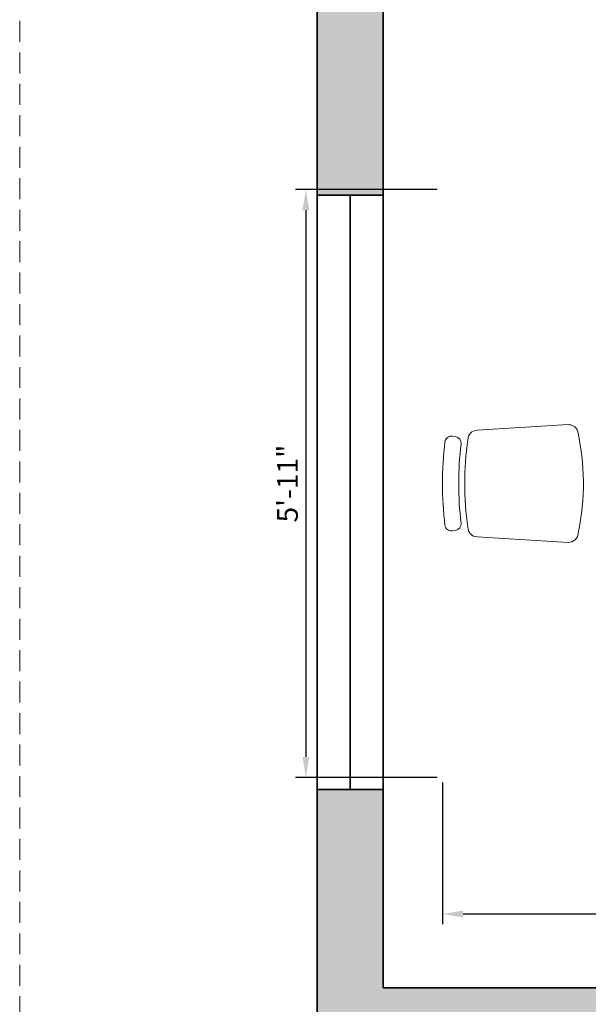
# Model space of a CAD drawing. Units: inches. Extents: x 1566 to 2546, y 1087 to 2705.
# Tile 7 of 27: x 1606 to 1674, y 1524 to 1643. Entities that reach past the tile are written whole.
import ezdxf

# ---------------------------------------------------------------- set-up
doc = ezdxf.new("R2010")
doc.units = ezdxf.units.IN
doc.linetypes.add('DASHED', pattern=[19.05, 12.7, -6.35])
for name, color, linetype, lineweight in [('A-ANNO-DIMS', 2, 'Continuous', 18), ('A-FLOR-OVHD', 8, 'DASHED', 18), ('A-FURN', 8, 'Continuous', 18), ('A-WALL', 7, 'Continuous', 35), ('A-WALL-PATT', 8, 'Continuous', 13)]:
    doc.layers.add(name, color=color, linetype=linetype, lineweight=lineweight)
doc.styles.get("Standard").update_dxf_attribs({"font": 'arial.ttf'})
doc.dimstyles.new('ISO-25', dxfattribs={"dimtxt": 2.5, "dimasz": 2.5, "dimexe": 1.25, "dimexo": 0.625, "dimtad": 1, "dimtxsty": 'Standard', "dimcen": 2.5, "dimadec": 0, "dimazin": 0, "dimtfac": 1, "dimtmove": 0, "dimatfit": 3, "dimfxl": 1, "dimarcsym": 0})

# ---------------------------------------------------------------- blocks, each defined once
blk = doc.blocks.new('A$C421907B3')
at = {"ltscale": 0.1}
for points in [[(0.77, 0.0782, -0.399285), (0.74, 0.1067), (0.7231, 0.3861, -0.305593), (0.7404, 0.4148, -0.109362), (1.0554, 0.4176, -0.429301), (1.0853, 0.3861), (1.0684, 0.1067, -0.399285), (1.0384, 0.0782, -0.071734)], [(0.9042, 0.05, 0.030867), (1.0261, 0.0575, -0.408428), (1.0484, 0.0405), (1.0498, 0.0306, -0.419966), (1.0325, 0.0079, -0.030916), (0.9042, 0, -0.030916), (0.7759, 0.0079, -0.419966), (0.7586, 0.0306), (0.76, 0.0405, -0.408428), (0.7823, 0.0575, 0.030867)]]:
    blk.add_lwpolyline(points, format="xyb", close=True, dxfattribs=at)
blk = doc.blocks.new('*D59')
at = {"layer": 'A-ANNO-DIMS', "color": 0, "lineweight": -2, "transparency": 16777216}
for p, q in [((1656.69, 1551.04), (1656.69, 1533.89)), ((1766.84, 1551.04), (1766.84, 1533.89)), ((1659.19, 1535.14), (1764.34, 1535.14))]:
    blk.add_line(p, q, dxfattribs=at)
at = {"layer": 'A-ANNO-DIMS', "color": 0, "transparency": 16777216}
for points in [[(1659.19, 1535.55), (1659.19, 1534.72), (1656.69, 1535.14)], [(1764.34, 1535.55), (1764.34, 1534.72), (1766.84, 1535.14)]]:
    blk.add_solid(points, dxfattribs=at)
at = {"layer": 'Defpoints', "color": 0, "transparency": 16777216}
for p in [(1656.69, 1551.66), (1766.84, 1551.66), (1766.84, 1535.14)]:
    blk.add_point(p, dxfattribs=at)
at = {"layer": 'A-ANNO-DIMS', "color": 0, "transparency": 16777216, "insert": (1711.76, 1537.06), "char_height": 2.5, "attachment_point": 5}
blk.add_mtext('DINING SET 9\'-2"', dxfattribs=at)
blk = doc.blocks.new('*D60')
at = {"layer": 'A-ANNO-DIMS', "color": 0, "lineweight": -2, "transparency": 16777216}
for p, q in [((1656.06, 1622.86), (1638.92, 1622.86)), ((1640.17, 1620.36), (1640.17, 1554.16)), ((1656.06, 1551.66), (1638.92, 1551.66))]:
    blk.add_line(p, q, dxfattribs=at)
at = {"layer": 'A-ANNO-DIMS', "color": 0, "transparency": 16777216}
for points in [[(1639.75, 1620.36), (1640.58, 1620.36), (1640.17, 1622.86)], [(1639.75, 1554.16), (1640.58, 1554.16), (1640.17, 1551.66)]]:
    blk.add_solid(points, dxfattribs=at)
at = {"layer": 'Defpoints', "color": 0, "transparency": 16777216}
for p in [(1656.69, 1622.86), (1640.17, 1551.66), (1656.69, 1551.66)]:
    blk.add_point(p, dxfattribs=at)
at = {"layer": 'A-ANNO-DIMS', "color": 0, "transparency": 16777216, "insert": (1638.26, 1587.26), "char_height": 2.5, "attachment_point": 5, "rotation": 90}
blk.add_mtext('5\'-11"', dxfattribs=at)

msp = doc.modelspace()

# ---------------------------------------------------------------- hatches: boundary and pattern name
at = {"layer": 'A-WALL-PATT'}
h = msp.add_hatch(color=256, dxfattribs=at)
h.dxf.hatch_style = 1
h.paths.add_polyline_path([(2001.53, 1778.2), (1641.53, 1778.2), (1641.53, 1746.2), (1649.53, 1746.2), (1649.53, 1770.2), (1769.53, 1770.2), (1769.53, 1650.2), (1767.53, 1650.2), (1767.53, 1648.2), (1767.53, 1646.2), (1819.53, 1646.2), (1819.53, 1650.2), (1773.53, 1650.2), (1773.53, 1770.2), (1941.53, 1770.2), (1941.53, 1756.2), (1945.53, 1756.2), (1945.53, 1770.2), (1993.53, 1770.2), (1993.53, 1650.2), (1945.53, 1650.2), (1945.53, 1652.2), (1943.53, 1652.2), (1941.53, 1652.2), (1941.53, 1650.2), (1867.53, 1650.2), (1867.53, 1642.2), (1871.53, 1642.2), (1871.53, 1646.2), (1993.53, 1646.2), (1993.53, 1526.2), (1871.53, 1526.2), (1871.53, 1606.2), (1867.53, 1606.2), (1867.53, 1522.2), (1993.53, 1522.2), (1993.53, 1387.2), (1959.53, 1387.2), (1959.53, 1397.2), (1955.53, 1397.2), (1955.53, 1387.2), (1903.53, 1387.2), (1903.53, 1383.2), (1993.53, 1383.2), (1993.53, 1364.3), (1993.53, 1211.2), (1939.53, 1211.2), (1939.53, 1203.2), (1993.53, 1203.2), (1993.53, 1154.2), (2001.53, 1154.2)])
h.paths.add_polyline_path([(1649.53, 1646.2), (1731.53, 1646.2), (1731.53, 1650.2), (1649.53, 1650.2), (1649.53, 1674.2), (1641.53, 1674.2), (1641.53, 1622.2), (1649.53, 1622.2)], flags=17)
h.paths.add_polyline_path([(1649.53, 1550.2), (1641.53, 1550.2), (1641.53, 1510.2), (1649.53, 1510.2), (1649.53, 1522.2), (1731.53, 1522.2), (1731.53, 1500.2), (1735.53, 1500.2), (1735.53, 1522.2), (1767.53, 1522.2), (1767.53, 1500.2), (1771.53, 1500.2), (1771.53, 1526.2), (1649.53, 1526.2)], flags=17)
h.paths.add_polyline_path([(1649.53, 1464.2), (1735.53, 1464.2), (1735.53, 1470.2), (1731.53, 1470.2), (1731.53, 1468.2), (1649.53, 1468.2), (1649.53, 1480.2), (1641.53, 1480.2), (1641.53, 1419.2), (1649.53, 1419.2)], flags=17)
h.paths.add_polyline_path([(1649.53, 1323.2), (1641.53, 1323.2), (1641.53, 1270.2), (1667.53, 1270.2), (1667.53, 1278.2), (1649.53, 1278.2)], flags=17)
h.paths.add_polyline_path([(1763.53, 1278.2), (1727.53, 1278.2), (1727.53, 1270.2), (1763.53, 1270.2)], flags=17)
h.paths.add_polyline_path([(1823.53, 1383.2), (1827.53, 1383.2), (1827.53, 1385.2), (1827.53, 1387.2), (1819.53, 1387.2), (1819.53, 1324.21), (1819.53, 1278.2), (1811.53, 1278.2), (1811.53, 1274.2), (1811.53, 1270.2), (1819.53, 1270.2), (1819.53, 1203.2), (1877.53, 1203.2), (1877.53, 1211.2), (1823.53, 1211.2)], flags=17)

# ---------------------------------------------------------------- linework, layer by layer
at = {"layer": 'A-FLOR-OVHD', "ltscale": 0.2}
msp.add_line((1605.53, 1130.2), (1605.53, 1778.2), dxfattribs=at)
at = {"layer": 'A-WALL'}
for p, q in [((1641.53, 1154.2), (1641.53, 1778.2)), ((1649.53, 1526.2), (1649.53, 1646.2)), ((1641.53, 1622.2), (1649.53, 1622.2)), ((1645.53, 1622.2), (1645.53, 1550.2)), ((1649.53, 1550.2), (1641.53, 1550.2)), ((1649.53, 1526.2), (1771.53, 1526.2))]:
    msp.add_line(p, q, dxfattribs=at)

# ---------------------------------------------------------------- block references
at = {"layer": 'A-FURN', "xscale": 39.3701, "yscale": 39.3701, "zscale": 39.3701, "rotation": 270.0000000000005}
msp.add_blockref('A$C421907B3', (1656.69, 1622.86), dxfattribs=at)

# ---------------------------------------------------------------- dimensions: what is measured, and where the dimension line sits
at = {"layer": 'A-ANNO-DIMS'}
dim = msp.add_linear_dim(base=(1640.17, 1551.66), p1=(1656.69, 1622.86), p2=(1656.69, 1551.66), angle=270, dimstyle='ISO-25', override={"dimdec": 1, "dimrnd": 0, "dimzin": 1, "dimlunit": 4, "dimfrac": 2}, dxfattribs=at)
dim.commit()
dim.dimension.update_dxf_attribs({"geometry": '*D60', "text_midpoint": (1638.26, 1587.26)})
dim = msp.add_linear_dim(base=(1766.8396, 1535.1383), p1=(1656.6889, 1551.6609), p2=(1766.8396, 1551.6609), angle=0, text='DINING SET <>', dimstyle='ISO-25', override={"dimdec": 1, "dimrnd": 0, "dimzin": 1, "dimlunit": 4, "dimfrac": 2}, dxfattribs=at)
dim.commit()
dim.dimension.update_dxf_attribs({"geometry": '*D59', "text_midpoint": (1711.7643, 1537.0559)})

doc.saveas('drawing.dxf')
